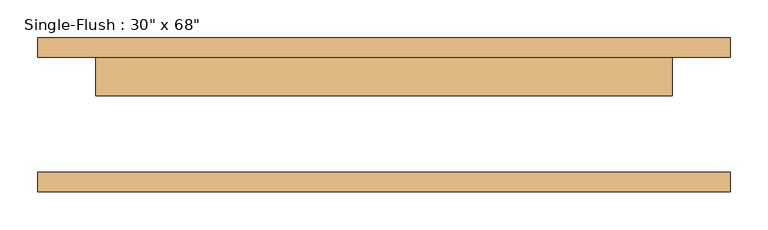
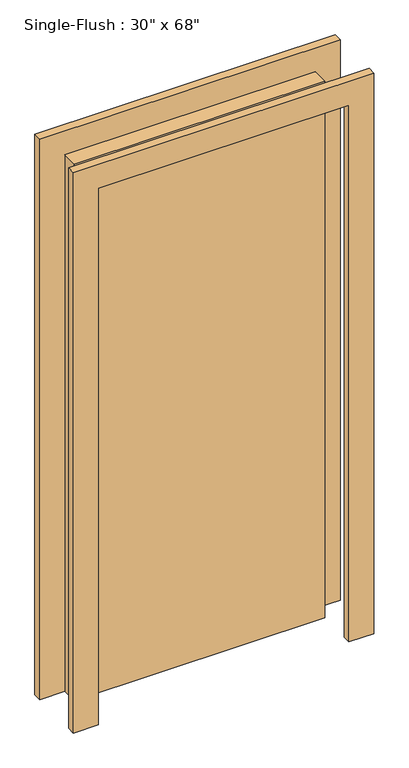
"""IFC4 building model written with IfcOpenShell, lengths in millimetres: door geometry."""

from ifc_helpers import new_model, si_unit, frame, origin, origin_with_axes, place, context, project, spatial, polyline, outline, extrude, source, transform, mapped, element, save


def door_1a1933ce(model_context):
    return source(origin(), model_context, "Body", "SweptSolid", [
        extrude(outline(polyline([(1803.4, -457.2), (0.0, -457.2), (0.0, -381.0), (1727.2, -381.0), (1727.2, 381.0), (0.0, 381.0), (0.0, 457.2), (1803.4, 457.2), (1803.4, -457.2)])), frame((0.0, 76.2, 0.0), z_axis=(0.0, 1.0, 0.0), x_axis=(0.0, 0.0, 1.0)), (0.0, 0.0, 1.0), 25.4),
        extrude(outline(polyline([(1803.4, 457.2), (1803.4, -457.2), (0.0, -457.2), (0.0, -381.0), (1727.2, -381.0), (1727.2, 381.0), (0.0, 381.0), (0.0, 457.2), (1803.4, 457.2)])), frame((0.0, -101.6, 0.0), z_axis=(0.0, 1.0, 0.0), x_axis=(0.0, 0.0, 1.0)), (0.0, 0.0, 1.0), 25.4),
        extrude(outline(polyline([(381.0, 25.4), (-381.0, 25.4), (-381.0, 76.2), (381.0, 76.2), (381.0, 25.4)])), origin_with_axes(), (0.0, 0.0, 1.0), 1727.2),
    ])


if __name__ == "__main__":
    model = new_model("IFC4")
    model_context = context("Model", 3, world=origin())
    ifc_project = project(units=[si_unit("LENGTHUNIT", "METRE", prefix="MILLI")], contexts=[model_context])
    site = spatial("IfcSite", under=ifc_project)
    building = spatial("IfcBuilding", under=site)
    placement = place(None, origin())
    door_shape = door_1a1933ce(model_context)
    element("IfcDoor", 1, ObjectType="Single-Flush : 30\" x 68\"", at=placement, inside=building, context=model_context, shape_type="MappedRepresentation", body=[
        mapped(door_shape, transform((0.0, 0.0, 0.0), x_axis=(1.0, 0.0, 0.0), y_axis=(0.0, 1.0, 0.0), z_axis=(0.0, 0.0, 1.0))),
    ])
    save(model, "model.ifc")

# Revit data of these elements
# Type "Single-Flush : 30\" x 68\""
#   Type Mark = "10"
#   Construction Type Id = "MDOOR"
#   Assembly Code = "C1020"
#   Analytic Construction = "Metal"
#   Thickness = 0' - 2"
#   Heat Transfer Coefficient (U) = 0.651978 BTU/(h·ft²·°F)
#   Height = 5' - 8"
#   Trim Projection Ext = 0' - 1"
#   Trim Projection Int = 0' - 1"
#   Trim Width = 0' - 3"
#   Width = 2' - 6"
#   Define Thermal Properties by = 1
#   Door Material = Door - Panel
#   Frame Material = Door - Frame
#   Visual Light Transmittance = 0
#   Solar Heat Gain Coefficient = 0
#   Function = (empty or 0)
#   Wall Closure = (empty or 0)
# Element 1 (IfcDoor, "Single-Flush : 30\" x 68\"")
#   Materials on its faces: "Door - Frame", "Door - Panel"
# Materials
#   "Door - Panel": class "Wood", colour RGB 210 159 95, transparency 0
#   "Door - Frame": colour RGB 118 70 51, transparency 0
